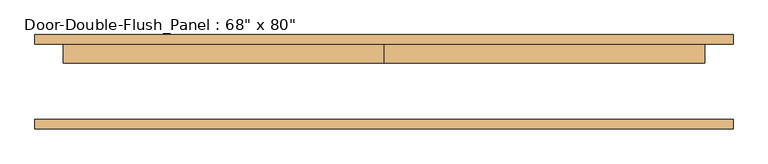
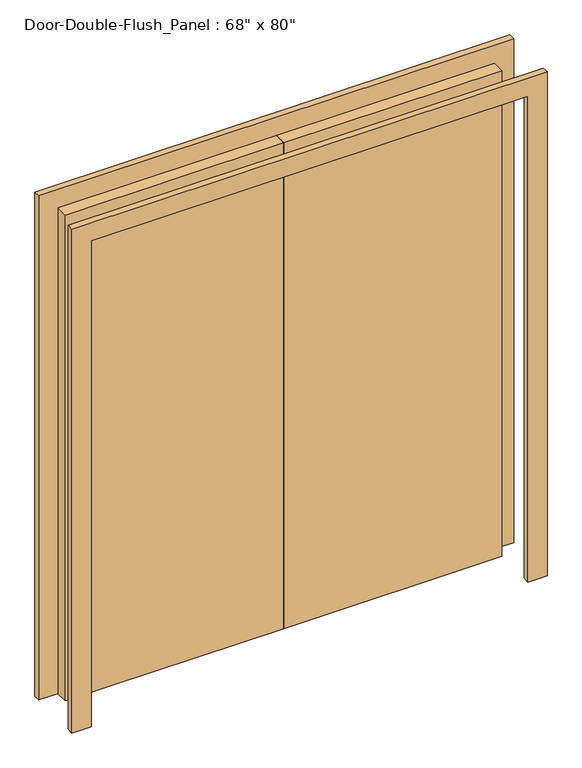
"""IFC4 building model written with IfcOpenShell, lengths in millimetres: door geometry."""

from ifc_helpers import new_model, si_unit, frame, origin, origin_with_axes, place, context, project, spatial, polyline, outline, extrude, source, transform, mapped, element, save


def door_aae36eb6(model_context):
    return source(origin(), model_context, "Body", "SweptSolid", [
        extrude(outline(polyline([(2032.0, -863.6), (2032.0, 863.6), (0.0, 863.6), (0.0, 939.8), (2108.2, 939.8), (2108.2, -939.8), (0.0, -939.8), (0.0, -863.6), (2032.0, -863.6)])), frame((0.0, -127.0, 0.0), z_axis=(0.0, 1.0, 0.0), x_axis=(0.0, 0.0, 1.0)), (0.0, 0.0, 1.0), 25.4),
        extrude(outline(polyline([(2032.0, -863.6), (2032.0, 863.6), (0.0, 863.6), (0.0, 939.8), (2108.2, 939.8), (2108.2, -939.8), (0.0, -939.8), (0.0, -863.6), (2032.0, -863.6)])), frame((0.0, 101.6, 0.0), z_axis=(0.0, 1.0, 0.0), x_axis=(0.0, 0.0, 1.0)), (0.0, 0.0, 1.0), 25.4),
        extrude(outline(polyline([(0.0, 101.6), (863.6, 101.6), (863.6, 50.8), (0.0, 50.8), (0.0, 101.6)])), origin_with_axes(), (0.0, 0.0, 1.0), 2032.0),
        extrude(outline(polyline([(-863.6, 101.6), (0.0, 101.6), (0.0, 50.8), (-863.6, 50.8), (-863.6, 101.6)])), origin_with_axes(), (0.0, 0.0, 1.0), 2032.0),
    ])


if __name__ == "__main__":
    model = new_model("IFC4")
    model_context = context("Model", 3, world=origin())
    ifc_project = project(units=[si_unit("LENGTHUNIT", "METRE", prefix="MILLI")], contexts=[model_context])
    site = spatial("IfcSite", under=ifc_project)
    building = spatial("IfcBuilding", under=site)
    placement = place(None, origin())
    door_shape = door_aae36eb6(model_context)
    element("IfcDoor", 1, ObjectType="Door-Double-Flush_Panel : 68\" x 80\"", at=placement, inside=building, context=model_context, shape_type="MappedRepresentation", body=[
        mapped(door_shape, transform((0.0, 0.0, 0.0), x_axis=(1.0, 0.0, 0.0), y_axis=(0.0, 1.0, 0.0), z_axis=(0.0, 0.0, 1.0))),
    ])
    save(model, "model.ifc")

# Revit data of these elements
# Type "Door-Double-Flush_Panel : 68\" x 80\""
#   Type Mark = "9"
#   Construction Type Id = "DOOR"
#   Assembly Code = "C1020"
#   Analytic Construction = "Wooden"
#   Thickness = 0' - 2"
#   Thermal Resistance (R) = 2.5876 (h·ft²·°F)/BTU
#   Swing Angle [instance default] = 90.00°
#   Panel Width = 2' - 10"
#   Heat Transfer Coefficient (U) = 0.3865 BTU/(h·ft²·°F)
#   Height = 6' - 8"
#   Trim Projection Ext = 0' - 1"
#   Trim Projection Int = 0' - 1"
#   Trim Width = 0' - 3"
#   Width = 5' - 8"
#   Define Thermal Properties by = 1
#   Panel Material = Wood - Birch - Solid Stained Light Low Gloss
#   Trim Material = Paint - Sienna
#   Visual Light Transmittance = 0
#   Solar Heat Gain Coefficient = 0
#   Function = (empty or 0)
#   Wall Closure = (empty or 0)
# Element 1 (IfcDoor, "Door-Double-Flush_Panel : 68\" x 80\"")
#   Materials on its faces: "Paint - Sienna", "Wood - Birch - Solid Stained Light Low Gloss"
# Materials
#   "Wood - Birch - Solid Stained Light Low Gloss": class "Wood", colour RGB 210 159 95, transparency 0, Cost = 0
#   "Paint - Sienna": colour RGB 118 70 51, transparency 0, Cost = 0
